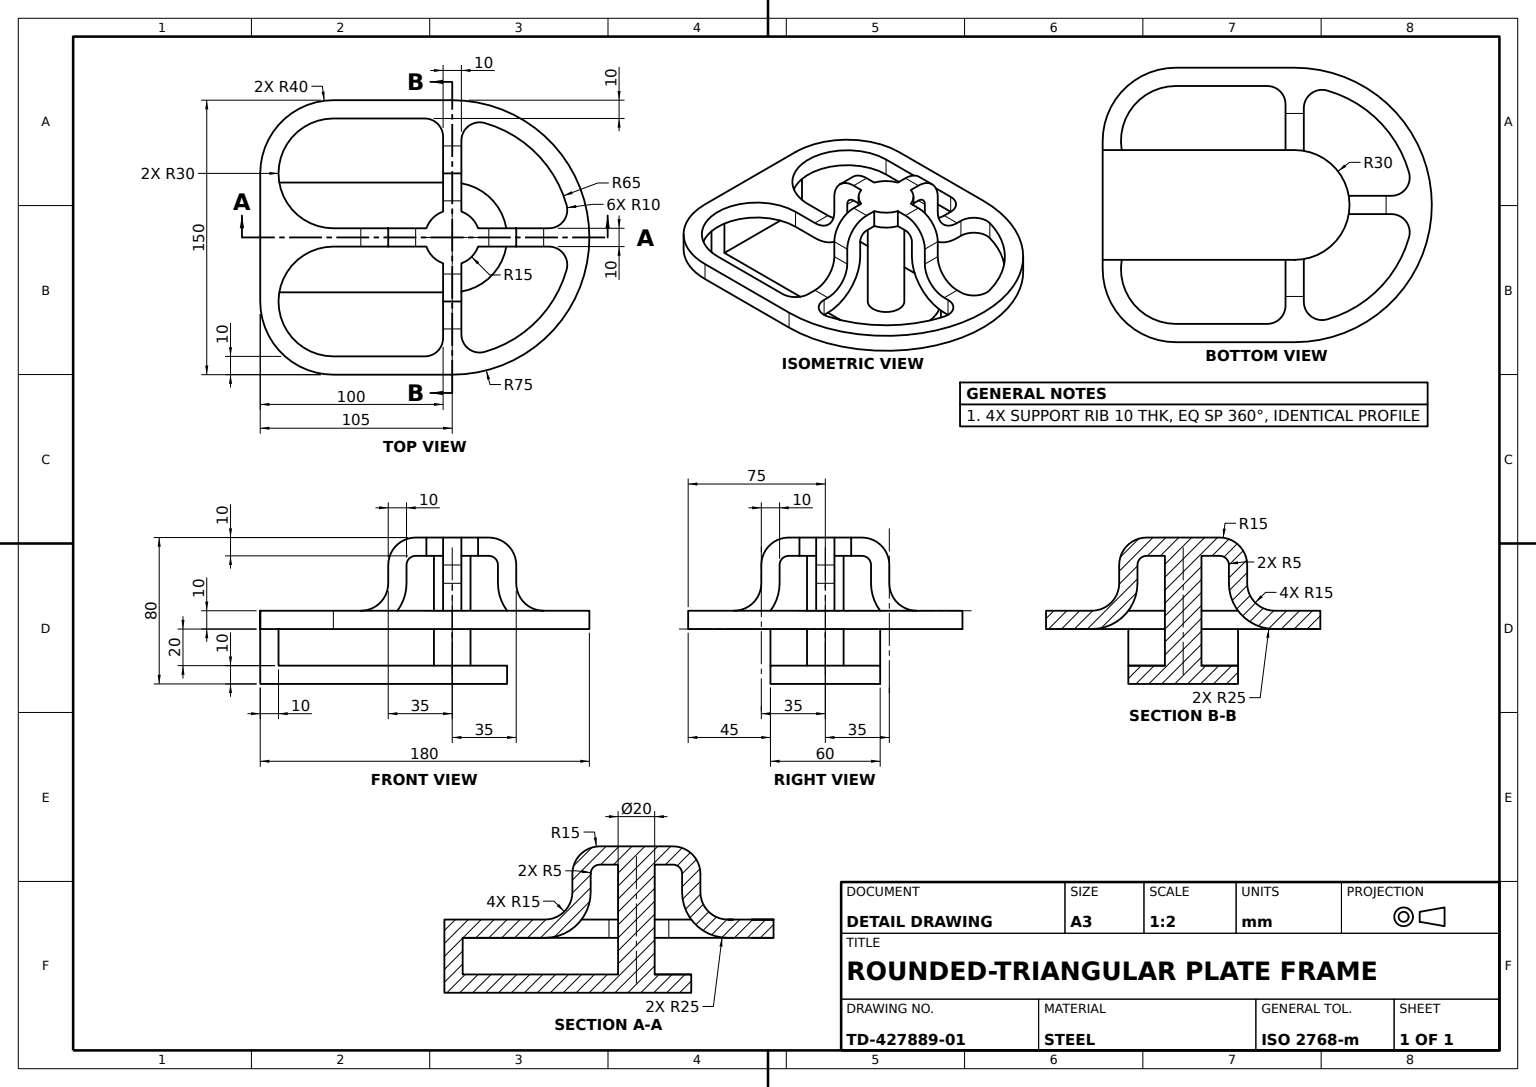
SolidWorks part; units mm, degrees
material "Plain Carbon Steel"
ref_plane "Front Plane" through (0, 0, 0) normal (0, 0, 1) x (1, 0, 0)
ref_plane "Top Plane" through (0, 0, 0) normal (0, 1, 0) x (1, 0, 0)
ref_plane "Right Plane" through (0, 0, 0) normal (1, 0, 0) x (0, 0, -1)
sketch "Central Post Sketch" plane through (0, 0, 0) normal (0, 1, 0) x (1, 0, 0)
  circle A0 centre (0, 0) radius 10
  dimension "D1" = 20
extrude "Central Post Ø20" add sketch "Central Post Sketch" along normal mid plane 80
sketch "Plate Outline Sketch" plane through (0, 0, 0) normal (0, 1, 0) x (1, 0, 0)
  line L0 (0, 0) -> (75, 0) construction
  line L1 (-65, 75) -> (0, 75)
  line L2 (-105, 35) -> (-105, -35)
  line L3 (-65, -75) -> (0, -75)
  arc A0 (-65, -75) -> (-105, -35) centre (-65, -35) cw
  arc A1 (-105, 35) -> (-65, 75) centre (-65, 35) cw
  arc A2 (0, -75) -> (0, 75) centre (0, 0) ccw
  point P11 (75, 75)
  dimension "D5" = 40
  dimension "D6" = 75
  dimension "D1" = 105
  dimension "D2" = 75
  dimension "D4" = 75
extrude "Mounting Plate" add sketch "Plate Outline Sketch" against normal blind 10
sketch "Plate Cutouts Sketch" plane through (0, 0, 0) normal (0, 1, 0) x (1, 0, 0)
  line L0 (8.6603, -5) -> (52.915, -5) construction
  line L1 (-5, -50) -> (-5, -55)
  line L2 (5, -50) -> (5, -52.915)
  line L3 (75, 0) -> (0, 0) construction
  line L4 (0, 65) -> (0, 0) construction
  line L5 (-5, 55) -> (-5, 50)
  line L6 (-65, -65) -> (0, -65)
  line L7 (0, 65) -> (-65, 65)
  line L8 (-95, 35) -> (-95, -35)
  line L9 (-65, -65) -> (-15, -65)
  line L10 (-15, 65) -> (-65, 65)
  line L14 (5, 52.915) -> (5, 50)
  line L15 (8.6603, 5) -> (52.915, 5) construction
  line L16 (-95, 35) -> (0, 35) construction
  line L17 (-95, -35) -> (0, -35) construction
  line L18 (-105, 35) -> (-105, -35) construction
  line L19 (-65, 5) -> (-65, -5)
  line L20 (-65, 0) -> (-105, 0) construction
  line L22 (52.915, 5) -> (52.915, -5)
  line L23 (-5, 50) -> (5, 50)
  line L24 (-5, -50) -> (5, -50)
  line L25 (0, -35) -> (0, -65) construction
  arc A5 (62.5359, 17.7273) -> (17.7273, 62.5359) centre (0, 0) ccw
  arc A6 (-95, -35) -> (-65, -65) centre (-65, -35) ccw
  arc A7 (0, -65) -> (0, 65) centre (0, 0) ccw
  arc A8 (-65, 65) -> (-95, 35) centre (-65, 35) ccw
  arc A9 (-65, -5) -> (-65, -65) centre (-65, -35) ccw
  arc A10 (17.7273, -62.5359) -> (62.5359, -17.7273) centre (0, 0) ccw
  arc A11 (-65, 65) -> (-65, 5) centre (-65, 35) ccw
  arc A12 (0, -75) -> (0, 75) centre (0, 0) ccw construction
  arc A13 (-5, -55) -> (-15, -65) centre (-15, -55) cw
  arc A14 (-5, 55) -> (-15, 65) centre (-15, 55) ccw
  arc A15 (5, -52.915) -> (17.7273, -62.5359) centre (15, -52.915) ccw
  arc A16 (52.915, -5) -> (62.5359, -17.7273) centre (52.915, -15) cw
  arc A17 (52.915, 5) -> (62.5359, 17.7273) centre (52.915, 15) ccw
  arc A18 (17.7273, 62.5359) -> (5, 52.915) centre (15, 52.915) ccw
  circle A21 centre (0, 0) radius 10 construction
  circle A22 centre (0, 0) radius 10
  point P42 (-5, -65)
  point P45 (-5, 65)
  point P49 (64.8074, -5)
  point P52 (64.8074, 5)
  circle M32 centre (0, 0) radius 10
  dimension "D4" = 10
  dimension "D5" = 10
  dimension "D2" = 5
  dimension "D3" = 10
  dimension "D1" = 10
sketch "Pad Sketch" plane through (0, -40, 0) normal (0, -1, 0) x (1, 0, 0)
  line L0 (-105, -35) -> (-105, 35) construction
  line L1 (-105, 30) -> (0, 30)
  line L2 (-105, 30) -> (-105, -30)
  line L3 (-105, -30) -> (0, -30)
  arc A2 (0, 30) -> (0, -30) centre (0, 0) cw
  point P6 (-105, 0)
  dimension "D3" = 30
  dimension "D1" = 60
extrude "Rectangular Pad 60x30" add sketch "Pad Sketch" against normal blind 10
sketch "Side Wall Sketch" plane through (0, 0, 0) normal (0, 0, 1) x (1, 0, 0)
  line L0 (0, -30) -> (-105, -30) construction
  line L1 (-105, -10) -> (-95, -10)
  line L2 (-105, -10) -> (-105, -30)
  line L3 (-105, -30) -> (-95, -30)
  line L4 (-95, -10) -> (-95, -30)
  dimension "D1" = 10
extrude "Side Wall" add sketch "Side Wall Sketch" along normal mid plane 60
sketch "Hub Sketch" plane through (0, 40, 0) normal (0, 1, 0) x (1, 0, 0)
  circle A0 centre (0, 0) radius 15
  dimension "D1" = 30
extrude "Hub Ø30" add sketch "Hub Sketch" against normal blind 10
sketch "Support Rib Sketch" plane through (0, 0, 0) normal (0, 0, 1) x (1, 0, 0)
  line L0 (0, 40) -> (-20, 40)
  line L1 (-35, 25) -> (-35, 15)
  line L2 (0, 30) -> (-20, 30)
  line L3 (-65, 0) -> (0, 0) construction
  line L4 (-25, 25) -> (-25, 15)
  line L6 (0, 40) -> (0, 30)
  line L7 (15, 40) -> (-15, 40) construction
  line L8 (-50, 0) -> (-65, 0)
  line L9 (-65, 0) -> (-65, -10)
  line L10 (-65, -10) -> (-50, -10)
  arc A0 (-20, 40) -> (-35, 25) centre (-20, 25) ccw
  arc A1 (-35, 15) -> (-50, 0) centre (-50, 15) cw
  arc A2 (-20, 30) -> (-25, 25) centre (-20, 25) ccw
  arc A3 (-25, 15) -> (-50, -10) centre (-50, 15) cw
  dimension "D2" = 15
  dimension "D3" = 15
  dimension "D1" = 35
  dimension "D4" = 10
extrude "Plate Cutouts" cut sketch "Plate Cutouts Sketch" against normal blind 10 contours A5 A18 L14 L23 L5 A14 L10 A11 L19 A9 L9 A13 L1 L24 L2 A15 A10 A16 L22 A17 M32
extrude "Support Rib" add sketch "Support Rib Sketch" along normal mid plane 10 contours A1 L8 L9 L10 A3 L4 A2 L2 L6 L0 A0 L1
pattern_circular "Rib Pattern 4x" count 4 over 360 about axis through (0, 0, 0) along (0, 1, 0) of "Support Rib"
